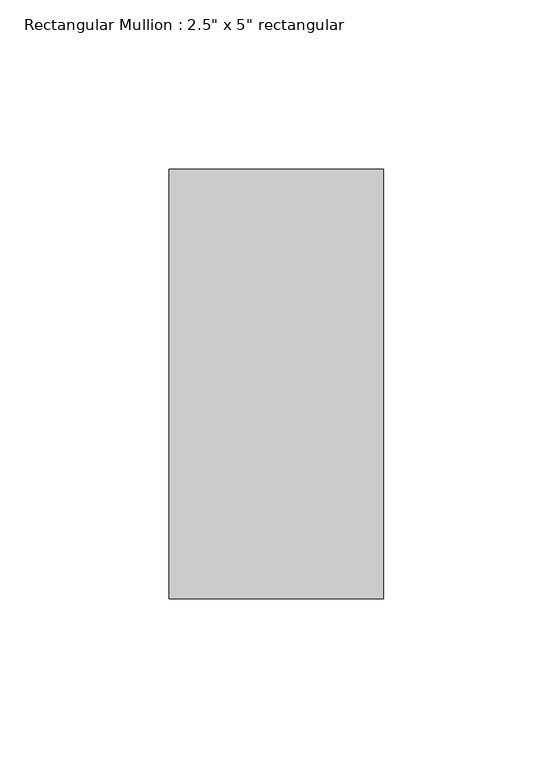
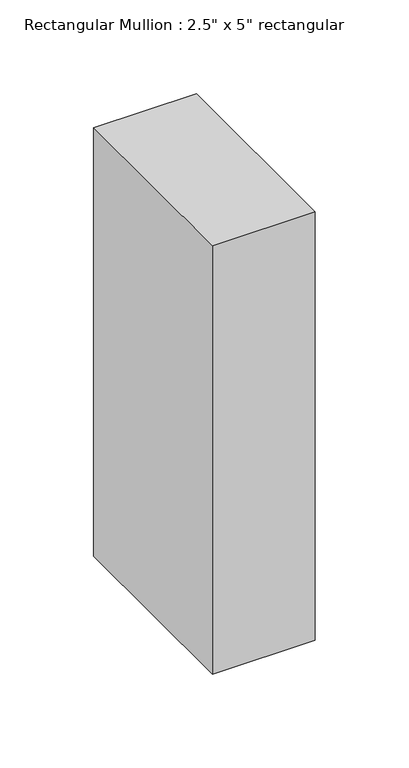
"""IFC4 building model written with IfcOpenShell, lengths in millimetres: member geometry."""

from ifc_helpers import new_model, si_unit, frame, origin, place, context, project, spatial, polyline, outline, extrude, source, transform, mapped, element, save


def member_6be37683(model_context):
    return source(origin(), model_context, "Body", "SweptSolid", [
        extrude(outline(polyline([(31.75, 63.5), (31.75, -63.5), (-31.75, -63.5), (-31.75, 63.5), (31.75, 63.5)])), frame((0.0, 0.0, -279.4), z_axis=(0.0, 0.0, 1.0), x_axis=(1.0, 0.0, 0.0)), (0.0, 0.0, 1.0), 279.4),
    ])


if __name__ == "__main__":
    model = new_model("IFC4")
    model_context = context("Model", 3, world=origin())
    ifc_project = project(units=[si_unit("LENGTHUNIT", "METRE", prefix="MILLI")], contexts=[model_context])
    site = spatial("IfcSite", under=ifc_project)
    building = spatial("IfcBuilding", under=site)
    placement = place(None, origin())
    member_shape = member_6be37683(model_context)
    element("IfcMember", 1, ObjectType="Rectangular Mullion : 2.5\" x 5\" rectangular", at=placement, inside=building, context=model_context, shape_type="MappedRepresentation", body=[
        mapped(member_shape, transform((0.0, 0.0, 0.0), x_axis=(1.0, 0.0, 0.0), y_axis=(0.0, 1.0, 0.0), z_axis=(0.0, 0.0, 1.0))),
    ])
    save(model, "model.ifc")

# Revit data of these elements
# Type "Rectangular Mullion : 2.5\" x 5\" rectangular"
#   built-in parameter 1007304 = 0.416667 (stored number, unit not read)
#   built-in parameter 1007301 = 0.104167 (stored number, unit not read)
#   built-in parameter 1007300 = 0.104167 (stored number, unit not read)
# Element 1 (IfcMember, "Rectangular Mullion : 2.5\" x 5\" rectangular")
#   Materials on its faces: "Aluminum"
# Materials
#   "Aluminum": class "Metal", colour RGB 247 247 247, transparency 0, Description = "Aluminum 6061", Cost = 0
